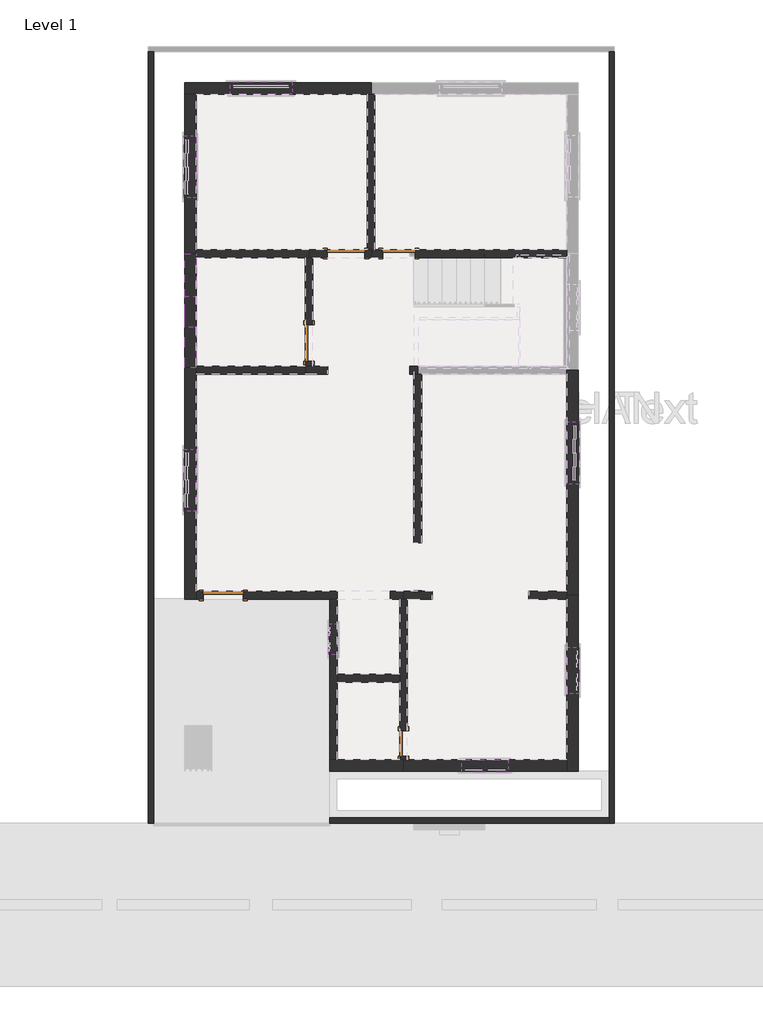
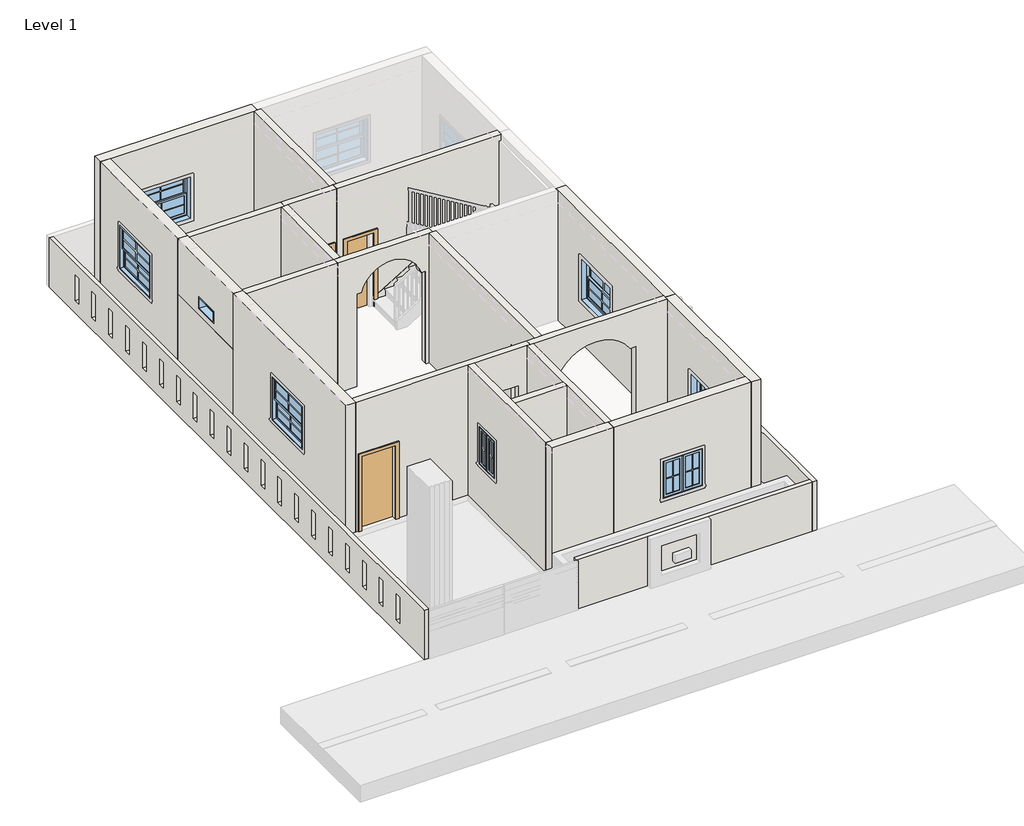
# One storey, part 1 of 3: 25 walls, 8 windows, 5 doors.
"""IFC4 building model written with IfcOpenShell, lengths in millimetres."""

from ifc_helpers import new_model, si_unit, frame, origin, origin_with_axes, place, context, project, spatial, polyline, circle_curve, outline, extrude, faceted_brep, transform, mapped, element, save
from ifc_brep_helpers import plane_surface, revolved_surface, advanced_brep
from components import door_85c31a06, door_fe267433, door_77f51d0b, door_a6948854, door_ee35e093, fixed_2_8c8825d0, window_casement_double_2_fb285ced, window_casement_double_3_90de19e9, window_double_hung_4_eadb0177, window_double_hung_4_aab3aae7

model = new_model("IFC4")

# Units and contexts
model_context = context("Model", 3, world=origin())
ifc_project = project(units=[si_unit("LENGTHUNIT", "METRE", prefix="MILLI")], contexts=[model_context])

# Site, building, storey
site = spatial("IfcSite", under=ifc_project)
building = spatial("IfcBuilding", under=site)
storey = spatial("IfcBuildingStorey", under=building, Name="Level 1", Elevation=0.0)

# Doors
placement = place(None, origin())
door_shape = door_85c31a06(model_context)
element("IfcDoor", 1, ObjectType="Single-Flush : 1'8\"", at=placement, inside=storey, context=model_context, shape_type="MappedRepresentation", body=[
    mapped(door_shape, transform((-1607.764062, -6283.5142637, 152.4), x_axis=(0.0, -1.0, 0.0), y_axis=(1.0, 0.0, 0.0), z_axis=(0.0, 0.0, 1.0))),
])
door_2_shape = door_fe267433(model_context)
element("IfcDoor", 2, ObjectType="Single-Flush : 2'1\"", at=placement, inside=storey, context=model_context, shape_type="MappedRepresentation", body=[
    mapped(door_2_shape, transform((-1696.664062, 3330.3857363, 152.4), x_axis=(-1.0, 0.0, 0.0), y_axis=(0.0, -1.0, 0.0), z_axis=(0.0, 0.0, 1.0))),
])
door_3_shape = door_77f51d0b(model_context)
element("IfcDoor", 3, ObjectType="Single-Flush : 2'4\"", at=placement, inside=storey, context=model_context, shape_type="MappedRepresentation", body=[
    mapped(door_3_shape, transform((-3461.964062, 1577.7857363, 152.4), x_axis=(0.0, -1.0, 0.0), y_axis=(1.0, 0.0, 0.0), z_axis=(0.0, 0.0, 1.0))),
])
door_4_shape = door_a6948854(model_context)
element("IfcDoor", 4, ObjectType="Single-Flush : 2'5\"", at=placement, inside=storey, context=model_context, shape_type="MappedRepresentation", body=[
    mapped(door_4_shape, transform((-2738.064062, 3330.3857363, 152.4), x_axis=(1.0, 0.0, 0.0), y_axis=(0.0, 1.0, 0.0), z_axis=(0.0, 0.0, 1.0))),
])
door_5_shape = door_ee35e093(model_context)
element("IfcDoor", 5, ObjectType="Single-Flush : 2'7\"", at=placement, inside=storey, context=model_context, shape_type="MappedRepresentation", body=[
    mapped(door_5_shape, transform((-5144.714062, -3375.2142637, 152.4), x_axis=(-1.0, 0.0, 0.0), y_axis=(0.0, -1.0, 0.0), z_axis=(0.0, 0.0, 1.0))),
])

# Walls
element("IfcWall", 6, ObjectType="Generic - 4\"", at=placement, inside=storey, context=model_context, shape_type="Brep", body=[
    faceted_brep([(2430.835938, 7292.7857363, 0.0), (2430.835938, -7744.0142637, 0.0), (2430.835938, -7845.6142637, 0.0), (2430.835938, -7845.6142637, 1219.2), (2430.835938, -7744.0142637, 1219.2), (2430.835938, 7292.7857363, 1219.2), (2532.435938, 7292.7857363, 0.0), (2532.435938, 7292.7857363, 1219.2), (2532.435938, -7845.6142637, 1219.2), (2532.435938, -7845.6142637, 0.0)], [[[0, 1, 2, 3, 4, 5]], [[6, 7, 8, 9]], [[2, 1, 0, 6, 9]], [[5, 4, 3, 8, 7]], [[0, 5, 7, 6]], [[3, 2, 9, 8]]]),
])
element("IfcWall", 7, ObjectType="Generic - 4\"", at=placement, inside=storey, context=model_context, shape_type="SweptSolid", body=[
    extrude(outline(polyline([(-3055.564062, -7744.0142637), (2430.835938, -7744.0142637), (2430.835938, -7845.6142637), (-3055.564062, -7845.6142637), (-3055.564062, -7744.0142637)])), origin_with_axes(), (0.0, 0.0, 1.0), 1219.2),
])
element("IfcWall", 8, ObjectType="Generic - 4\"", at=placement, inside=storey, context=model_context, shape_type="SweptSolid", body=[
    extrude(outline(polyline([(7292.7857363, 0.0), (-7845.6142637, 0.0), (-7845.6142637, 1219.2), (7292.7857363, 1219.2), (7292.7857363, 0.0)]), holes=[polyline([(6243.785737, 939.8), (6102.415296, 939.8), (6102.415296, 304.8), (6243.785737, 304.8), (6243.785737, 939.8)]), polyline([(-6722.914263, 939.8), (-6864.284704, 939.8), (-6864.284704, 304.8), (-6722.914263, 304.8), (-6722.914263, 939.8)]), polyline([(-6040.4563683, 939.8), (-6181.8268093, 939.8), (-6181.8268093, 304.8), (-6040.4563683, 304.8), (-6040.4563683, 939.8)]), polyline([(-5357.9984735, 939.8), (-5499.3689146, 939.8), (-5499.3689146, 304.8), (-5357.9984735, 304.8), (-5357.9984735, 939.8)]), polyline([(-4675.5405788, 939.8), (-4816.9110198, 939.8), (-4816.9110198, 304.8), (-4675.5405788, 304.8), (-4675.5405788, 939.8)]), polyline([(-3993.0826841, 939.8), (-4134.4531251, 939.8), (-4134.4531251, 304.8), (-3993.0826841, 304.8), (-3993.0826841, 939.8)]), polyline([(-3310.6247893, 939.8), (-3451.9952303, 939.8), (-3451.9952303, 304.8), (-3310.6247893, 304.8), (-3310.6247893, 939.8)]), polyline([(-2628.1668946, 939.8), (-2769.5373356, 939.8), (-2769.5373356, 304.8), (-2628.1668946, 304.8), (-2628.1668946, 939.8)]), polyline([(-1945.7089999, 939.8), (-2087.0794409, 939.8), (-2087.0794409, 304.8), (-1945.7089999, 304.8), (-1945.7089999, 939.8)]), polyline([(-1263.2511051, 939.8), (-1404.6215461, 939.8), (-1404.6215461, 304.8), (-1263.2511051, 304.8), (-1263.2511051, 939.8)]), polyline([(-580.7932104, 939.8), (-722.1636514, 939.8), (-722.1636514, 304.8), (-580.7932104, 304.8), (-580.7932104, 939.8)]), polyline([(101.6646844, 939.8), (-39.7057567, 939.8), (-39.7057567, 304.8), (101.6646844, 304.8), (101.6646844, 939.8)]), polyline([(784.1225791, 939.8), (642.7521381, 939.8), (642.7521381, 304.8), (784.1225791, 304.8), (784.1225791, 939.8)]), polyline([(1466.5804738, 939.8), (1325.2100328, 939.8), (1325.2100328, 304.8), (1466.5804738, 304.8), (1466.5804738, 939.8)]), polyline([(2149.0383686, 939.8), (2007.6679276, 939.8), (2007.6679276, 304.8), (2149.0383686, 304.8), (2149.0383686, 939.8)]), polyline([(2831.4962633, 939.8), (2690.1258223, 939.8), (2690.1258223, 304.8), (2831.4962633, 304.8), (2831.4962633, 939.8)]), polyline([(3513.954158, 939.8), (3372.583717, 939.8), (3372.583717, 304.8), (3513.954158, 304.8), (3513.954158, 939.8)]), polyline([(4196.4120528, 939.8), (4055.0416118, 939.8), (4055.0416118, 304.8), (4196.4120528, 304.8), (4196.4120528, 939.8)]), polyline([(4878.8699475, 939.8), (4737.4995065, 939.8), (4737.4995065, 304.8), (4878.8699475, 304.8), (4878.8699475, 939.8)]), polyline([(5561.3278422, 939.8), (5419.9574012, 939.8), (5419.9574012, 304.8), (5561.3278422, 304.8), (5561.3278422, 939.8)])]), frame((-6611.564062, 0.0, 0.0), z_axis=(1.0, 0.0, 0.0), x_axis=(0.0, 1.0, 0.0)), (0.0, 0.0, 1.0), 101.6),
])
element("IfcWall", 9, ObjectType="Generic - 6\"", at=placement, inside=storey, context=model_context, shape_type="Brep", body=[
    faceted_brep([(-2318.964062, 6454.5857363, 152.4), (-2318.964062, 3406.5857363, 152.4), (-2318.964062, 3406.5857363, 3352.8), (-2318.964062, 6454.5857363, 3352.8), (-2166.564062, 6454.5857363, 152.4), (-2166.564062, 6454.5857363, 3352.8), (-2166.564062, 3406.5857363, 3352.8), (-2166.564062, 3406.5857363, 152.4), (-2242.764062, 6454.5857363, 152.4), (-2242.764062, 3406.5857363, 152.4), (-2242.764062, 3406.5857363, 3352.8), (-2242.764062, 6454.5857363, 3352.8)], [[[0, 1, 2, 3]], [[4, 5, 6, 7]], [[1, 0, 8, 4, 7, 9]], [[3, 2, 10, 6, 5, 11]], [[0, 3, 11, 5, 4, 8]], [[2, 1, 9, 7, 6, 10]]]),
])
element("IfcWall", 10, ObjectType="Generic - 6\"", at=placement, inside=storey, context=model_context, shape_type="Brep", body=[
    faceted_brep([(-5671.764062, 3254.1857363, 3352.8), (-5671.764062, 3254.1857363, 152.4), (-3538.164062, 3254.1857363, 152.4), (-3461.964062, 3254.1857363, 152.4), (-3461.964062, 3254.1857363, 3352.8), (-3538.164062, 3254.1857363, 3352.8), (-5671.764062, 3406.5857363, 152.4), (-5671.764062, 3406.5857363, 3352.8), (-3461.964062, 3406.5857363, 3352.8), (-3461.964062, 3406.5857363, 152.4), (-5671.764062, 3330.3857363, 152.4), (-5671.764062, 3330.3857363, 3352.8)], [[[0, 1, 2, 3, 4, 5]], [[6, 7, 8, 9]], [[3, 2, 1, 10, 6, 9]], [[4, 3, 9, 8]], [[0, 5, 4, 8, 7, 11]], [[0, 11, 7, 6, 10, 1]]]),
])
element("IfcWall", 11, ObjectType="Generic - 6\"", at=placement, inside=storey, context=model_context, shape_type="Brep", body=[
    faceted_brep([(-5671.764062, 968.1857363, 152.4), (-3538.164062, 968.1857363, 152.4), (-3538.164062, 968.1857363, 3352.8), (-5671.764062, 968.1857363, 3352.8), (-5671.764062, 1120.5857363, 152.4), (-5671.764062, 1120.5857363, 3352.8), (-3538.164062, 1120.5857363, 3352.8), (-3538.164062, 1120.5857363, 152.4), (-5671.764062, 1095.1857363, 152.4), (-5671.764062, 1095.1857363, 3352.8)], [[[0, 1, 2, 3]], [[4, 5, 6, 7]], [[1, 0, 8, 4, 7]], [[2, 1, 7, 6]], [[3, 2, 6, 5, 9]], [[0, 3, 9, 5, 4, 8]]]),
])
element("IfcWall", 12, ObjectType="Generic - 6\"", at=placement, inside=storey, context=model_context, shape_type="Brep", body=[
    faceted_brep([(-1404.564062, 968.1857363, 152.4), (-1404.564062, -2346.4297845, 152.4), (-1404.564062, -2346.4297845, 2616.2), (-1404.564062, -3288.7710229, 2616.2), (-1404.564062, -3288.7710229, 152.4), (-1404.564062, -3299.0142637, 152.4), (-1404.564062, -3299.0142637, 3352.8), (-1404.564062, 968.1857363, 3352.8), (-1252.164062, -2346.4297845, 152.4), (-1252.164062, 968.1857363, 152.4), (-1252.164062, 968.1857363, 3352.8), (-1252.164062, -3299.0142637, 3352.8), (-1252.164062, -3299.0142637, 152.4), (-1252.164062, -3288.7710229, 152.4), (-1252.164062, -3288.7710229, 2616.2), (-1252.164062, -2346.4297845, 2616.2), (-1328.364062, 968.1857363, 152.4), (-1328.364062, 968.1857363, 3352.8)], [[[0, 1, 2, 3, 4, 5, 6, 7]], [[8, 9, 10, 11, 12, 13, 14, 15]], [[6, 5, 12, 11]], [[1, 0, 16, 9, 8]], [[7, 6, 11, 10, 17]], [[2, 1, 8, 15]], [[3, 2, 15, 14]], [[4, 3, 14, 13]], [[5, 4, 13, 12]], [[0, 7, 17, 10, 9, 16]]]),
])
element("IfcWall", 13, ObjectType="Generic - 6\"", at=placement, inside=storey, context=model_context, shape_type="Brep", body=[
    faceted_brep([(-2903.164062, -3451.4142637, 2438.4), (-1865.8319448, -3451.4142637, 2438.4), (-1865.8319448, -3451.4142637, 152.4), (-1683.964062, -3451.4142637, 152.4), (-1607.764062, -3451.4142637, 152.4), (-1607.764062, -3451.4142637, 3352.8), (-1683.964062, -3451.4142637, 3352.8), (-2903.164062, -3451.4142637, 3352.8), (-3055.564062, -3451.4142637, 3352.8), (-5671.764062, -3451.4142637, 3352.8), (-5671.764062, -3451.4142637, 152.4), (-5538.414062, -3451.4142637, 152.4), (-5538.414062, -3451.4142637, 1981.2), (-4751.014062, -3451.4142637, 1981.2), (-4751.014062, -3451.4142637, 152.4), (-3055.564062, -3451.4142637, 152.4), (-2903.164062, -3451.4142637, 152.4), (-1865.8319448, -3299.0142637, 2438.4), (-2903.164062, -3299.0142637, 2438.4), (-2903.164062, -3299.0142637, 152.4), (-4751.014062, -3299.0142637, 152.4), (-4751.014062, -3299.0142637, 1981.2), (-5538.414062, -3299.0142637, 1981.2), (-5538.414062, -3299.0142637, 152.4), (-5671.764062, -3299.0142637, 152.4), (-5671.764062, -3299.0142637, 3352.8), (-1607.764062, -3299.0142637, 3352.8), (-1607.764062, -3299.0142637, 152.4), (-1865.8319448, -3299.0142637, 152.4)], [[[0, 1, 2, 3, 4, 5, 6, 7, 8, 9, 10, 11, 12, 13, 14, 15, 16]], [[17, 18, 19, 20, 21, 22, 23, 24, 25, 26, 27, 28]], [[17, 1, 0, 18]], [[1, 17, 28, 2]], [[22, 12, 11, 23]], [[12, 22, 21, 13]], [[13, 21, 20, 14]], [[10, 24, 23, 11]], [[27, 4, 3, 2, 28]], [[19, 16, 15, 14, 20]], [[5, 4, 27, 26]], [[9, 8, 7, 6, 5, 26, 25]], [[10, 9, 25, 24]], [[18, 0, 16, 19]]]),
])
element("IfcWall", 14, ObjectType="Generic - 6\"", at=placement, inside=storey, context=model_context, shape_type="Brep", body=[
    faceted_brep([(-3055.564062, -3451.4142637, 152.4), (-3055.564062, -6601.0142637, 152.4), (-3055.564062, -6601.0142637, 3352.8), (-3055.564062, -3451.4142637, 3352.8), (-3055.564062, -3934.0142637, 2133.6), (-3055.564062, -4543.6142637, 2133.6), (-3055.564062, -4543.6142637, 1219.2), (-3055.564062, -3934.0142637, 1219.2), (-2903.164062, -3451.4142637, 152.4), (-2903.164062, -3451.4142637, 2438.4), (-2903.164062, -3451.4142637, 3352.8), (-2903.164062, -4924.6142637, 3352.8), (-2903.164062, -5077.0142637, 3352.8), (-2903.164062, -6601.0142637, 3352.8), (-2903.164062, -6601.0142637, 152.4), (-2903.164062, -5077.0142637, 152.4), (-2903.164062, -4924.6142637, 152.4), (-2903.164062, -3934.0142637, 2133.6), (-2903.164062, -3934.0142637, 1219.2), (-2903.164062, -4543.6142637, 1219.2), (-2903.164062, -4543.6142637, 2133.6)], [[[0, 1, 2, 3], [4, 5, 6, 7]], [[8, 9, 10, 11, 12, 13, 14, 15, 16], [17, 18, 19, 20]], [[1, 0, 8, 16, 15, 14]], [[3, 2, 13, 12, 11, 10]], [[2, 1, 14, 13]], [[18, 17, 4, 7]], [[19, 18, 7, 6]], [[20, 19, 6, 5]], [[17, 20, 5, 4]], [[0, 3, 10, 9, 8]]]),
])
element("IfcWall", 15, ObjectType="Generic - 6\"", at=placement, inside=storey, context=model_context, shape_type="Brep", body=[
    faceted_brep([(-1683.964062, -6601.0142637, 3352.8), (-1683.964062, -5077.0142637, 3352.8), (-1683.964062, -4924.6142637, 3352.8), (-1683.964062, -3451.4142637, 3352.8), (-1683.964062, -3451.4142637, 152.4), (-1683.964062, -4924.6142637, 152.4), (-1683.964062, -5077.0142637, 152.4), (-1683.964062, -6029.5142637, 152.4), (-1683.964062, -6029.5142637, 1981.2), (-1683.964062, -6537.5142637, 1981.2), (-1683.964062, -6537.5142637, 152.4), (-1683.964062, -6601.0142637, 152.4), (-1531.564062, -3451.4142637, 3352.8), (-1531.564062, -6601.0142637, 3352.8), (-1531.564062, -6601.0142637, 152.4), (-1531.564062, -6537.5142637, 152.4), (-1531.564062, -6537.5142637, 1981.2), (-1531.564062, -6029.5142637, 1981.2), (-1531.564062, -6029.5142637, 152.4), (-1531.564062, -3451.4142637, 152.4), (-1607.764062, -6601.0142637, 152.4), (-1607.764062, -3451.4142637, 152.4), (-1607.764062, -6601.0142637, 3352.8), (-1607.764062, -3451.4142637, 3352.8)], [[[0, 1, 2, 3, 4, 5, 6, 7, 8, 9, 10, 11]], [[12, 13, 14, 15, 16, 17, 18, 19]], [[14, 20, 11, 10, 15]], [[4, 21, 19, 18, 7, 6, 5]], [[3, 2, 1, 0, 22, 13, 12, 23]], [[9, 16, 15, 10]], [[16, 9, 8, 17]], [[17, 8, 7, 18]], [[0, 11, 20, 14, 13, 22]], [[4, 3, 23, 12, 19, 21]]]),
])
element("IfcWall", 16, ObjectType="Generic - 6\"", at=placement, inside=storey, context=model_context, shape_type="SweptSolid", body=[
    extrude(outline(polyline([(-1683.964062, -5077.0142637), (-2903.164062, -5077.0142637), (-2903.164062, -4924.6142637), (-1683.964062, -4924.6142637), (-1683.964062, -5077.0142637)])), frame((0.0, 0.0, 152.4), z_axis=(0.0, 0.0, 1.0), x_axis=(1.0, 0.0, 0.0)), (0.0, 0.0, 1.0), 3200.4),
])
element("IfcWall", 17, ObjectType="Generic - 6\"", at=placement, inside=storey, context=model_context, shape_type="Brep", body=[
    faceted_brep([(-3538.164062, 1120.5857363, 3352.8), (-3538.164062, 3254.1857363, 3352.8), (-3538.164062, 3254.1857363, 152.4), (-3538.164062, 1933.3857363, 152.4), (-3538.164062, 1933.3857363, 1981.2), (-3538.164062, 1222.1857363, 1981.2), (-3538.164062, 1222.1857363, 152.4), (-3538.164062, 1120.5857363, 152.4), (-3385.764062, 3254.1857363, 3352.8), (-3385.764062, 1120.5857363, 3352.8), (-3385.764062, 1120.5857363, 152.4), (-3385.764062, 1222.1857363, 152.4), (-3385.764062, 1222.1857363, 1981.2), (-3385.764062, 1933.3857363, 1981.2), (-3385.764062, 1933.3857363, 152.4), (-3385.764062, 3254.1857363, 152.4), (-3461.964062, 3254.1857363, 152.4), (-3461.964062, 3254.1857363, 3352.8)], [[[0, 1, 2, 3, 4, 5, 6, 7]], [[8, 9, 10, 11, 12, 13, 14, 15]], [[10, 7, 6, 11]], [[2, 16, 15, 14, 3]], [[1, 0, 9, 8, 17]], [[0, 7, 10, 9]], [[12, 5, 4, 13]], [[13, 4, 3, 14]], [[5, 12, 11, 6]], [[2, 1, 17, 8, 15, 16]]]),
])
element("IfcWall", 18, ObjectType="Generic - 6\"", at=placement, inside=storey, context=model_context, shape_type="Brep", body=[
    faceted_brep([(-2242.764062, 3254.1857363, 152.4), (-2014.164062, 3254.1857363, 152.4), (-2014.164062, 3254.1857363, 1981.2), (-1379.164062, 3254.1857363, 1981.2), (-1379.164062, 3254.1857363, 152.4), (1541.835938, 3254.1857363, 152.4), (1592.635938, 3254.1857363, 152.4), (1592.635938, 3254.1857363, 3352.8), (-2242.764062, 3254.1857363, 3352.8), (-2014.164062, 3406.5857363, 1981.2), (-2014.164062, 3406.5857363, 152.4), (-2166.564062, 3406.5857363, 152.4), (-2242.764062, 3406.5857363, 152.4), (-2242.764062, 3406.5857363, 3352.8), (-2166.564062, 3406.5857363, 3352.8), (1592.635938, 3406.5857363, 3352.8), (1592.635938, 3406.5857363, 152.4), (-1379.164062, 3406.5857363, 152.4), (-1379.164062, 3406.5857363, 1981.2), (1592.635938, 3330.3857363, 152.4), (1592.635938, 3330.3857363, 3352.8)], [[[0, 1, 2, 3, 4, 5, 6, 7, 8]], [[9, 10, 11, 12, 13, 14, 15, 16, 17, 18]], [[17, 16, 19, 6, 5, 4]], [[12, 11, 10, 1, 0]], [[8, 7, 20, 15, 14, 13]], [[0, 8, 13, 12]], [[4, 3, 18, 17]], [[3, 2, 9, 18]], [[2, 1, 10, 9]], [[6, 19, 16, 15, 20, 7]]]),
])
element("IfcWall", 19, ObjectType="Generic - 6\"", at=placement, inside=storey, context=model_context, shape_type="AdvancedBrep", body=[
    advanced_brep(
    [(1592.635938, -3451.4142637, 3352.8), (-1531.564062, -3451.4142637, 3352.8), (-1607.764062, -3451.4142637, 3352.8), (-1607.764062, -3451.4142637, 152.4), (-1531.564062, -3451.4142637, 152.4), (-1042.9877715, -3451.4142637, 152.4), (-1042.9877715, -3451.4142637, 2438.4), (-909.3649468, -3451.4142637, 2438.4), (732.5205767, -3451.4142637, 2438.4), (852.655246, -3451.4142637, 2438.4), (852.655246, -3451.4142637, 152.4), (1592.635938, -3451.4142637, 152.4), (-1607.764062, -3299.0142637, 3352.8), (-1404.564062, -3299.0142637, 3352.8), (-1252.164062, -3299.0142637, 3352.8), (1592.635938, -3299.0142637, 3352.8), (1592.635938, -3299.0142637, 152.4), (852.655246, -3299.0142637, 152.4), (852.655246, -3299.0142637, 2438.4), (732.5205767, -3299.0142637, 2438.4), (-909.3649468, -3299.0142637, 2438.4), (-1042.9877715, -3299.0142637, 2438.4), (-1042.9877715, -3299.0142637, 152.4), (-1252.164062, -3299.0142637, 152.4), (-1404.564062, -3299.0142637, 152.4), (-1607.764062, -3299.0142637, 152.4), (1592.635938, -3375.2142637, 3352.8), (1592.635938, -3375.2142637, 152.4)],
    [
        (0, 1),
        (1, 2),
        (2, 3),
        (3, 4),
        (4, 5),
        (5, 6),
        (6, 7),
        (7, 8, circle_curve(frame((-88.4221851, -3451.4142637, 1902.6141821), z_axis=(0.0, 1.0, 0.0), x_axis=(-1.0, 0.0, 0.0)), 980.3129402)),
        (8, 9),
        (9, 10),
        (10, 11),
        (11, 0),
        (12, 13),
        (13, 14),
        (14, 15),
        (15, 16),
        (16, 17),
        (17, 18),
        (18, 19),
        (19, 20, circle_curve(frame((-88.4221851, -3299.0142637, 1902.6141821), z_axis=(0.0, -1.0, 0.0), x_axis=(-1.0, 0.0, 0.0)), 980.3129402)),
        (20, 21),
        (21, 22),
        (22, 23),
        (23, 24),
        (24, 25),
        (25, 12),
        (0, 26),
        (26, 15),
        (12, 2),
        (9, 18),
        (17, 10),
        (5, 22),
        (21, 6),
        (7, 20),
        (19, 8),
        (3, 25),
        (16, 27),
        (27, 11),
    ],
    [
        plane_surface(frame((1706.935938, -3451.4142637, 3352.8), z_axis=(0.0, -1.0, 0.0), x_axis=(-1.0, 0.0, 0.0))),
        plane_surface(frame((1706.935938, -3299.0142637, 3352.8), z_axis=(0.0, 1.0, 0.0), x_axis=(1.0, 0.0, 0.0))),
        plane_surface(frame((1706.935938, -3451.4142637, 3352.8), z_axis=(0.0, 0.0, 1.0), x_axis=(0.0, 1.0, 0.0))),
        plane_surface(frame((852.655246, -3451.4142637, 2177.180621), z_axis=(-1.0, 0.0, 0.0), x_axis=(0.0, 1.0, 0.0))),
        plane_surface(frame((-1042.9877715, -3451.4142637, 487.9784957), z_axis=(1.0, 0.0, 0.0), x_axis=(0.0, 1.0, 0.0))),
        revolved_surface(polyline([(-1068.7351253, -3299.0142637, 1902.6141821), (-1068.7351253, -3451.4142637, 1902.6141821)]), (-88.4221851, -3299.0142637, 1902.6141821), (0.0, 1.0, 0.0)),
        plane_surface(frame((-1607.764062, -3451.4142637, 152.4), z_axis=(0.0, 0.0, -1.0), x_axis=(0.0, 1.0, 0.0))),
        plane_surface(frame((456.9071606, -3451.4142637, 152.4), z_axis=(0.0, 0.0, -1.0), x_axis=(0.0, 1.0, 0.0))),
        plane_surface(frame((-1607.764062, -3451.4142637, 3352.8), z_axis=(-1.0, 0.0, 0.0), x_axis=(0.0, 1.0, 0.0))),
        plane_surface(frame((1592.635938, 6454.5857363, 152.4), z_axis=(1.0, 0.0, 0.0), x_axis=(0.0, -1.0, 0.0))),
        plane_surface(frame((-1042.9877715, -3299.0142637, 2438.4), z_axis=(0.0, 0.0, -1.0), x_axis=(-1.0, 0.0, 0.0))),
    ],
    [
        (0, [[1, 2, 3, 4, 5, 6, 7, 8, 9, 10, 11, 12]]),
        (1, [[13, 14, 15, 16, 17, 18, 19, 20, 21, 22, 23, 24, 25, 26]]),
        (2, [[-2, -1, 27, 28, -15, -14, -13, 29]]),
        (3, [[30, -18, 31, -10]]),
        (4, [[32, -22, 33, -6]]),
        (5, [[-8, 34, -20, 35]]),
        (6, [[36, -25, -24, -23, -32, -5, -4]]),
        (7, [[37, 38, -11, -31, -17]]),
        (8, [[-3, -29, -26, -36]]),
        (9, [[-12, -38, -37, -16, -28, -27]]),
        (10, [[-33, -21, -34, -7]]),
        (10, [[-30, -9, -35, -19]]),
    ],
),
])
element("IfcWall", 20, ObjectType="Generic - 6\"", at=placement, inside=storey, context=model_context, shape_type="Brep", body=[
    faceted_brep([(-2369.764062, 3254.1857363, 1981.2), (-2369.764062, 3254.1857363, 152.4), (-2242.764062, 3254.1857363, 152.4), (-2242.764062, 3254.1857363, 3352.8), (-3385.764062, 3254.1857363, 3352.8), (-3461.964062, 3254.1857363, 3352.8), (-3461.964062, 3254.1857363, 152.4), (-3385.764062, 3254.1857363, 152.4), (-3106.364062, 3254.1857363, 152.4), (-3106.364062, 3254.1857363, 1981.2), (-2242.764062, 3406.5857363, 152.4), (-2318.964062, 3406.5857363, 152.4), (-2369.764062, 3406.5857363, 152.4), (-2369.764062, 3406.5857363, 1981.2), (-3106.364062, 3406.5857363, 1981.2), (-3106.364062, 3406.5857363, 152.4), (-3461.964062, 3406.5857363, 152.4), (-3461.964062, 3406.5857363, 3352.8), (-2318.964062, 3406.5857363, 3352.8), (-2242.764062, 3406.5857363, 3352.8)], [[[0, 1, 2, 3, 4, 5, 6, 7, 8, 9]], [[10, 11, 12, 13, 14, 15, 16, 17, 18, 19]], [[2, 1, 12, 11, 10]], [[8, 7, 6, 16, 15]], [[3, 2, 10, 19]], [[5, 4, 3, 19, 18, 17]], [[6, 5, 17, 16]], [[15, 14, 9, 8]], [[14, 13, 0, 9]], [[13, 12, 1, 0]]]),
])
element("IfcWall", 21, ObjectType="Generic - 6\"", at=placement, inside=storey, context=model_context, shape_type="AdvancedBrep", body=[
    advanced_brep(
    [(-1328.364062, 968.1857363, 3352.8), (-1404.564062, 968.1857363, 3352.8), (-3538.164062, 968.1857363, 3352.8), (-3538.164062, 968.1857363, 152.4), (-3088.5741654, 968.1857363, 152.4), (-3088.5741654, 968.1857363, 2438.4), (-2990.069581, 968.1857363, 2438.4), (-1595.0493956, 968.1857363, 2438.4), (-1480.764062, 968.1857363, 2438.4), (-1480.764062, 968.1857363, 152.4), (-1404.564062, 968.1857363, 152.4), (-1328.364062, 968.1857363, 152.4), (-3538.164062, 1120.5857363, 3352.8), (-3385.764062, 1120.5857363, 3352.8), (-1328.364062, 1120.5857363, 3352.8), (-1328.364062, 1120.5857363, 152.4), (-1480.764062, 1120.5857363, 152.4), (-1480.764062, 1120.5857363, 2438.4), (-1595.0493956, 1120.5857363, 2438.4), (-2990.069581, 1120.5857363, 2438.4), (-3088.5741654, 1120.5857363, 2438.4), (-3088.5741654, 1120.5857363, 152.4), (-3385.764062, 1120.5857363, 152.4), (-3538.164062, 1120.5857363, 152.4)],
    [
        (0, 1),
        (1, 2),
        (2, 3),
        (3, 4),
        (4, 5),
        (5, 6),
        (6, 7, circle_curve(frame((-2292.5594883, 968.1857363, 2260.6), z_axis=(0.0, 1.0, 0.0), x_axis=(-1.0, 0.0, 0.0)), 719.8146771)),
        (7, 8),
        (8, 9),
        (9, 10),
        (10, 11),
        (11, 0),
        (12, 13),
        (13, 14),
        (14, 15),
        (15, 16),
        (16, 17),
        (17, 18),
        (18, 19, circle_curve(frame((-2292.5594883, 1120.5857363, 2260.6), z_axis=(0.0, -1.0, 0.0), x_axis=(-1.0, 0.0, 0.0)), 719.8146771)),
        (19, 20),
        (20, 21),
        (21, 22),
        (22, 23),
        (23, 12),
        (6, 19),
        (18, 7),
        (15, 11),
        (9, 16),
        (0, 14),
        (12, 2),
        (3, 23),
        (21, 4),
        (5, 20),
        (17, 8),
    ],
    [
        plane_surface(frame((-3012.3741654, 968.1857363, 2260.6), z_axis=(0.0, -1.0, 0.0), x_axis=(0.0, 0.0, 1.0))),
        plane_surface(frame((-3012.3741654, 1120.5857363, 2260.6), z_axis=(0.0, 1.0, 0.0), x_axis=(0.0, 0.0, -1.0))),
        revolved_surface(polyline([(-3012.3741654, 1120.5857363, 2260.6), (-3012.3741654, 968.1857363, 2260.6)]), (-2292.5594883, 1120.5857363, 2260.6), (0.0, 1.0, 0.0)),
        plane_surface(frame((-1572.7448112, 968.1857363, 152.4), z_axis=(0.0, 0.0, -1.0), x_axis=(0.0, 1.0, 0.0))),
        plane_surface(frame((-1328.364062, 968.1857363, 3352.8), z_axis=(0.0, 0.0, 1.0), x_axis=(0.0, 1.0, 0.0))),
        plane_surface(frame((-3538.164062, 968.1857363, 152.4), z_axis=(0.0, 0.0, -1.0), x_axis=(0.0, 1.0, 0.0))),
        plane_surface(frame((-1328.364062, 968.1857363, 152.4), z_axis=(1.0, 0.0, 0.0), x_axis=(0.0, 1.0, 0.0))),
        plane_surface(frame((-3538.164062, 968.1857363, 3352.8), z_axis=(-1.0, 0.0, 0.0), x_axis=(0.0, 1.0, 0.0))),
        plane_surface(frame((-3088.5741654, 1120.5857363, 2438.4), z_axis=(0.0, 0.0, -1.0), x_axis=(-1.0, 0.0, 0.0))),
        plane_surface(frame((-3088.5741654, 1120.5857363, 2438.4), z_axis=(1.0, 0.0, 0.0), x_axis=(0.0, 0.0, -1.0))),
        plane_surface(frame((-1480.764062, 968.1857363, 2438.4), z_axis=(-1.0, 0.0, 0.0), x_axis=(0.0, 0.0, -1.0))),
    ],
    [
        (0, [[1, 2, 3, 4, 5, 6, 7, 8, 9, 10, 11, 12]]),
        (1, [[13, 14, 15, 16, 17, 18, 19, 20, 21, 22, 23, 24]]),
        (2, [[-7, 25, -19, 26]]),
        (3, [[27, -11, -10, 28, -16]]),
        (4, [[-2, -1, 29, -14, -13, 30]]),
        (5, [[31, -23, -22, 32, -4]]),
        (6, [[-12, -27, -15, -29]]),
        (7, [[-3, -30, -24, -31]]),
        (8, [[33, -20, -25, -6]]),
        (8, [[34, -8, -26, -18]]),
        (9, [[-33, -5, -32, -21]]),
        (10, [[-34, -17, -28, -9]]),
    ],
),
])
element("IfcWall", 22, ObjectType="Generic - 9\"", at=placement, inside=storey, context=model_context, shape_type="Brep", body=[
    faceted_brep([(-5900.364062, 6454.5857363, 152.4), (-5671.764062, 6454.5857363, 152.4), (-2318.964062, 6454.5857363, 152.4), (-2242.764062, 6454.5857363, 152.4), (-2242.764062, 6454.5857363, 3352.8), (-2318.964062, 6454.5857363, 3352.8), (-5671.764062, 6454.5857363, 3352.8), (-5900.364062, 6454.5857363, 3352.8), (-3792.164062, 6454.5857363, 2286.0), (-3792.164062, 6454.5857363, 1219.2), (-5011.364062, 6454.5857363, 1219.2), (-5011.364062, 6454.5857363, 2286.0), (-5900.364062, 6683.1857363, 152.4), (-5900.364062, 6683.1857363, 3352.8), (-2242.764062, 6683.1857363, 3352.8), (-2242.764062, 6683.1857363, 152.4), (-3792.164062, 6683.1857363, 2286.0), (-5011.364062, 6683.1857363, 2286.0), (-5011.364062, 6683.1857363, 1219.2), (-3792.164062, 6683.1857363, 1219.2)], [[[0, 1, 2, 3, 4, 5, 6, 7], [8, 9, 10, 11]], [[12, 13, 14, 15], [16, 17, 18, 19]], [[3, 2, 1, 0, 12, 15]], [[4, 3, 15, 14]], [[7, 6, 5, 4, 14, 13]], [[0, 7, 13, 12]], [[9, 8, 16, 19]], [[10, 9, 19, 18]], [[11, 10, 18, 17]], [[8, 11, 17, 16]]]),
])
element("IfcWall", 23, ObjectType="Generic - 9\"", at=placement, inside=storey, context=model_context, shape_type="Brep", body=[
    faceted_brep([(1592.635938, -6601.0142637, 152.4), (-1531.564062, -6601.0142637, 152.4), (-1607.764062, -6601.0142637, 152.4), (-1607.764062, -6601.0142637, 3352.8), (-1531.564062, -6601.0142637, 3352.8), (1592.635938, -6601.0142637, 3352.8), (-464.764062, -6601.0142637, 2133.6), (-464.764062, -6601.0142637, 1219.2), (449.635938, -6601.0142637, 1219.2), (449.635938, -6601.0142637, 2133.6), (1592.635938, -6829.6142637, 152.4), (1592.635938, -6829.6142637, 3352.8), (-1607.764062, -6829.6142637, 3352.8), (-1607.764062, -6829.6142637, 152.4), (-464.764062, -6829.6142637, 2133.6), (449.635938, -6829.6142637, 2133.6), (449.635938, -6829.6142637, 1219.2), (-464.764062, -6829.6142637, 1219.2)], [[[0, 1, 2, 3, 4, 5], [6, 7, 8, 9]], [[10, 11, 12, 13], [14, 15, 16, 17]], [[2, 1, 0, 10, 13]], [[3, 2, 13, 12]], [[5, 4, 3, 12, 11]], [[0, 5, 11, 10]], [[7, 6, 14, 17]], [[8, 7, 17, 16]], [[9, 8, 16, 15]], [[6, 9, 15, 14]]]),
])
element("IfcWall", 24, ObjectType="Generic - 9\"", at=placement, inside=storey, context=model_context, shape_type="Brep", body=[
    faceted_brep([(-5900.364062, 6454.5857363, 152.4), (-5900.364062, 3330.3857363, 152.4), (-5900.364062, 3330.3857363, 1981.2), (-5900.364062, 3330.3857363, 3352.8), (-5900.364062, 6454.5857363, 3352.8), (-5900.364062, 4422.5857363, 2286.0), (-5900.364062, 4422.5857363, 1219.2), (-5900.364062, 5641.7857363, 1219.2), (-5900.364062, 5641.7857363, 2286.0), (-5671.764062, 6454.5857363, 152.4), (-5671.764062, 6454.5857363, 3352.8), (-5671.764062, 3406.5857363, 3352.8), (-5671.764062, 3330.3857363, 3352.8), (-5671.764062, 3330.3857363, 152.4), (-5671.764062, 3406.5857363, 152.4), (-5671.764062, 4422.5857363, 2286.0), (-5671.764062, 5641.7857363, 2286.0), (-5671.764062, 5641.7857363, 1219.2), (-5671.764062, 4422.5857363, 1219.2)], [[[0, 1, 2, 3, 4], [5, 6, 7, 8]], [[9, 10, 11, 12, 13, 14], [15, 16, 17, 18]], [[1, 0, 9, 14, 13]], [[4, 3, 12, 11, 10]], [[0, 4, 10, 9]], [[6, 5, 15, 18]], [[7, 6, 18, 17]], [[8, 7, 17, 16]], [[5, 8, 16, 15]], [[1, 13, 12, 3, 2]]]),
])
element("IfcWall", 25, ObjectType="Generic - 9\"", at=placement, inside=storey, context=model_context, shape_type="Brep", body=[
    faceted_brep([(-5900.364062, 3330.3857363, 152.4), (-5900.364062, 1095.1857363, 152.4), (-5900.364062, 1095.1857363, 1981.2), (-5900.364062, 3330.3857363, 1981.2), (-5671.764062, 3330.3857363, 152.4), (-5671.764062, 3330.3857363, 1981.2), (-5671.764062, 1095.1857363, 1981.2), (-5671.764062, 1095.1857363, 152.4), (-5671.764062, 3254.1857363, 152.4)], [[[0, 1, 2, 3]], [[4, 5, 6, 7, 8]], [[1, 0, 4, 8, 7]], [[2, 1, 7, 6]], [[3, 2, 6, 5]], [[0, 3, 5, 4]]]),
])
element("IfcWall", 26, ObjectType="Generic - 9\"", at=placement, inside=storey, context=model_context, shape_type="Brep", body=[
    faceted_brep([(-1607.764062, -6601.0142637, 152.4), (-1683.964062, -6601.0142637, 152.4), (-2903.164062, -6601.0142637, 152.4), (-3055.564062, -6601.0142637, 152.4), (-3055.564062, -6601.0142637, 3352.8), (-2903.164062, -6601.0142637, 3352.8), (-1683.964062, -6601.0142637, 3352.8), (-1607.764062, -6601.0142637, 3352.8), (-1607.764062, -6829.6142637, 152.4), (-1607.764062, -6829.6142637, 3352.8), (-3055.564062, -6829.6142637, 3352.8), (-3055.564062, -6829.6142637, 152.4)], [[[0, 1, 2, 3, 4, 5, 6, 7]], [[8, 9, 10, 11]], [[3, 2, 1, 0, 8, 11]], [[7, 6, 5, 4, 10, 9]], [[0, 7, 9, 8]], [[4, 3, 11, 10]]]),
])
element("IfcWall", 27, ObjectType="Generic - 9\"", at=placement, inside=storey, context=model_context, shape_type="Brep", body=[
    faceted_brep([(1592.635938, 1044.3857363, 3352.8), (1592.635938, 1044.3857363, 152.4), (1592.635938, 993.5857363, 152.4), (1592.635938, 968.1857363, 152.4), (1592.635938, -3299.0142637, 152.4), (1592.635938, -3375.2142637, 152.4), (1592.635938, -3375.2142637, 3352.8), (1592.635938, -3299.0142637, 3352.8), (1592.635938, 968.1857363, 3352.8), (1592.635938, 28.3857363, 2286.0), (1592.635938, -1190.8142637, 2286.0), (1592.635938, -1190.8142637, 1219.2), (1592.635938, 28.3857363, 1219.2), (1821.235938, 1044.3857363, 152.4), (1821.235938, 1044.3857363, 3352.8), (1821.235938, -3375.2142637, 3352.8), (1821.235938, -3375.2142637, 152.4), (1821.235938, 28.3857363, 2286.0), (1821.235938, 28.3857363, 1219.2), (1821.235938, -1190.8142637, 1219.2), (1821.235938, -1190.8142637, 2286.0)], [[[0, 1, 2, 3, 4, 5, 6, 7, 8], [9, 10, 11, 12]], [[13, 14, 15, 16], [17, 18, 19, 20]], [[5, 4, 3, 2, 1, 13, 16]], [[6, 5, 16, 15]], [[0, 8, 7, 6, 15, 14]], [[17, 20, 10, 9]], [[20, 19, 11, 10]], [[19, 18, 12, 11]], [[18, 17, 9, 12]], [[0, 14, 13, 1]]]),
])
element("IfcWall", 28, ObjectType="Generic - 9\"", at=placement, inside=storey, context=model_context, shape_type="Brep", body=[
    faceted_brep([(1592.635938, -3375.2142637, 152.4), (1592.635938, -3451.4142637, 152.4), (1592.635938, -6601.0142637, 152.4), (1592.635938, -6829.6142637, 152.4), (1592.635938, -6829.6142637, 3352.8), (1592.635938, -6601.0142637, 3352.8), (1592.635938, -3451.4142637, 3352.8), (1592.635938, -3375.2142637, 3352.8), (1592.635938, -5305.6142637, 2133.6), (1592.635938, -5305.6142637, 1219.2), (1592.635938, -4391.2142637, 1219.2), (1592.635938, -4391.2142637, 2133.6), (1821.235938, -3375.2142637, 152.4), (1821.235938, -3375.2142637, 3352.8), (1821.235938, -6829.6142637, 3352.8), (1821.235938, -6829.6142637, 152.4), (1821.235938, -5305.6142637, 2133.6), (1821.235938, -4391.2142637, 2133.6), (1821.235938, -4391.2142637, 1219.2), (1821.235938, -5305.6142637, 1219.2)], [[[0, 1, 2, 3, 4, 5, 6, 7], [8, 9, 10, 11]], [[12, 13, 14, 15], [16, 17, 18, 19]], [[3, 2, 1, 0, 12, 15]], [[7, 6, 5, 4, 14, 13]], [[0, 7, 13, 12]], [[4, 3, 15, 14]], [[8, 11, 17, 16]], [[11, 10, 18, 17]], [[10, 9, 19, 18]], [[9, 8, 16, 19]]]),
])
element("IfcWall", 29, ObjectType="Generic - 9\"", at=placement, inside=storey, context=model_context, shape_type="Brep", body=[
    faceted_brep([(-5900.364062, 1095.1857363, 3352.8), (-5900.364062, 1095.1857363, 1981.2), (-5900.364062, 1095.1857363, 152.4), (-5900.364062, -3451.4142637, 152.4), (-5900.364062, -3451.4142637, 3352.8), (-5900.364062, -1724.2142637, 2286.0), (-5900.364062, -1724.2142637, 1219.2), (-5900.364062, -505.0142637, 1219.2), (-5900.364062, -505.0142637, 2286.0), (-5671.764062, 1095.1857363, 152.4), (-5671.764062, 1095.1857363, 1981.2), (-5671.764062, 1095.1857363, 3352.8), (-5671.764062, 968.1857363, 3352.8), (-5671.764062, -3299.0142637, 3352.8), (-5671.764062, -3451.4142637, 3352.8), (-5671.764062, -3451.4142637, 152.4), (-5671.764062, -3299.0142637, 152.4), (-5671.764062, 968.1857363, 152.4), (-5671.764062, -1724.2142637, 2286.0), (-5671.764062, -505.0142637, 2286.0), (-5671.764062, -505.0142637, 1219.2), (-5671.764062, -1724.2142637, 1219.2)], [[[0, 1, 2, 3, 4], [5, 6, 7, 8]], [[9, 10, 11, 12, 13, 14, 15, 16, 17], [18, 19, 20, 21]], [[3, 2, 9, 17, 16, 15]], [[0, 4, 14, 13, 12, 11]], [[4, 3, 15, 14]], [[5, 8, 19, 18]], [[8, 7, 20, 19]], [[7, 6, 21, 20]], [[6, 5, 18, 21]], [[0, 11, 10, 9, 2, 1]]]),
])
element("IfcWall", 30, ObjectType="Generic - 9\"", at=placement, inside=storey, context=model_context, shape_type="Brep", body=[
    faceted_brep([(-5900.364062, 3330.3857363, 1981.2), (-5900.364062, 1095.1857363, 1981.2), (-5900.364062, 1095.1857363, 3352.8), (-5900.364062, 3330.3857363, 3352.8), (-5900.364062, 1882.5857363, 2438.4), (-5900.364062, 1882.5857363, 2133.6), (-5900.364062, 2492.1857363, 2133.6), (-5900.364062, 2492.1857363, 2438.4), (-5671.764062, 3330.3857363, 1981.2), (-5671.764062, 3330.3857363, 3352.8), (-5671.764062, 3254.1857363, 3352.8), (-5671.764062, 1095.1857363, 3352.8), (-5671.764062, 1095.1857363, 1981.2), (-5671.764062, 1882.5857363, 2438.4), (-5671.764062, 2492.1857363, 2438.4), (-5671.764062, 2492.1857363, 2133.6), (-5671.764062, 1882.5857363, 2133.6)], [[[0, 1, 2, 3], [4, 5, 6, 7]], [[8, 9, 10, 11, 12], [13, 14, 15, 16]], [[1, 0, 8, 12]], [[2, 1, 12, 11]], [[3, 2, 11, 10, 9]], [[0, 3, 9, 8]], [[4, 7, 14, 13]], [[7, 6, 15, 14]], [[6, 5, 16, 15]], [[5, 4, 13, 16]]]),
])

# Windows
fixed_2_shape = fixed_2_8c8825d0(model_context)
element("IfcWindow", 31, ObjectType="Fixed : 2'", at=placement, inside=storey, context=model_context, shape_type="MappedRepresentation", body=[
    mapped(fixed_2_shape, transform((-5786.064062, 2149.2857363, 1219.2), x_axis=(0.0, -1.0, 0.0), y_axis=(1.0, 0.0, 0.0), z_axis=(0.0, 0.0, 1.0))),
])
window_casement_double_2_shape = window_casement_double_2_fb285ced(model_context)
element("IfcWindow", 32, ObjectType="Window-Casement-Double : 2'", at=placement, inside=storey, context=model_context, shape_type="MappedRepresentation", body=[
    mapped(window_casement_double_2_shape, transform((-2979.364062, -4238.8142637, 304.8), x_axis=(0.0, 1.0, 0.0), y_axis=(-1.0, 0.0, 0.0), z_axis=(0.0, 0.0, 1.0))),
])
window_casement_double_3_shape = window_casement_double_3_90de19e9(model_context)
element("IfcWindow", 33, ObjectType="Window-Casement-Double : 3'", at=placement, inside=storey, context=model_context, shape_type="MappedRepresentation", body=[
    mapped(window_casement_double_3_shape, transform((1706.935938, -4848.4142637, 304.8), x_axis=(0.0, -1.0, 0.0), y_axis=(1.0, 0.0, 0.0), z_axis=(0.0, 0.0, 1.0))),
])
element("IfcWindow", 34, ObjectType="Window-Casement-Double : 3'", at=placement, inside=storey, context=model_context, shape_type="MappedRepresentation", body=[
    mapped(window_casement_double_3_shape, transform((-7.564062, -6715.3142637, 304.8), x_axis=(-1.0, 0.0, 0.0), y_axis=(0.0, -1.0, 0.0), z_axis=(0.0, 0.0, 1.0))),
])
window_double_hung_4_shape = window_double_hung_4_eadb0177(model_context)
element("IfcWindow", 35, ObjectType="Window-Double-Hung : 4'", at=placement, inside=storey, context=model_context, shape_type="MappedRepresentation", body=[
    mapped(window_double_hung_4_shape, transform((-5786.064062, 5032.1857363, 304.8), x_axis=(0.0, 1.0, 0.0), y_axis=(-1.0, 0.0, 0.0), z_axis=(0.0, 0.0, 1.0))),
])
element("IfcWindow", 36, ObjectType="Window-Double-Hung : 4'", at=placement, inside=storey, context=model_context, shape_type="MappedRepresentation", body=[
    mapped(window_double_hung_4_shape, transform((1706.935938, -581.2142637, 304.8), x_axis=(0.0, -1.0, 0.0), y_axis=(1.0, 0.0, 0.0), z_axis=(0.0, 0.0, 1.0))),
])
element("IfcWindow", 37, ObjectType="Window-Double-Hung : 4'", at=placement, inside=storey, context=model_context, shape_type="MappedRepresentation", body=[
    mapped(window_double_hung_4_shape, transform((-5786.064062, -1114.6142637, 304.8), x_axis=(0.0, 1.0, 0.0), y_axis=(-1.0, 0.0, 0.0), z_axis=(0.0, 0.0, 1.0))),
])
window_double_hung_4_2_shape = window_double_hung_4_aab3aae7(model_context)
element("IfcWindow", 38, ObjectType="Window-Double-Hung : 4'", at=placement, inside=storey, context=model_context, shape_type="MappedRepresentation", body=[
    mapped(window_double_hung_4_2_shape, transform((-4401.764062, 6568.8857363, 304.8), x_axis=(-1.0, 0.0, 0.0), y_axis=(0.0, -1.0, 0.0), z_axis=(0.0, 0.0, 1.0))),
])

save(model, "model.ifc")

# Revit data of these elements
# Type "Single-Flush : 1'8\""
#   Type Mark = "11"
#   Construction Type Id = "MDOOR"
#   Assembly Code = "C1020"
#   Analytic Construction = "Metal"
#   Thickness = 0' - 2"
#   Heat Transfer Coefficient (U) = 0.651978 BTU/(h·ft²·°F)
#   Height = 6' - 0"
#   Trim Projection Ext = 0' - 1"
#   Trim Projection Int = 0' - 1"
#   Trim Width = 0' - 3"
#   Width = 1' - 8"
#   Define Thermal Properties by = 1
#   Door Material = Door - Panel
#   Frame Material = Door - Frame
#   Visual Light Transmittance = 0
#   Solar Heat Gain Coefficient = 0
#   Function = (empty or 0)
#   Wall Closure = (empty or 0)
# Type "Single-Flush : 2'1\""
#   Type Mark = "9"
#   Construction Type Id = "MDOOR"
#   Assembly Code = "C1020"
#   Analytic Construction = "Metal"
#   Thickness = 0' - 2"
#   Heat Transfer Coefficient (U) = 0.651978 BTU/(h·ft²·°F)
#   Height = 6' - 0"
#   Trim Projection Ext = 0' - 1"
#   Trim Projection Int = 0' - 1"
#   Trim Width = 0' - 3"
#   Width = 2' - 1"
#   Define Thermal Properties by = 1
#   Door Material = Door - Panel
#   Frame Material = Door - Frame
#   Visual Light Transmittance = 0
#   Solar Heat Gain Coefficient = 0
#   Function = (empty or 0)
#   Wall Closure = (empty or 0)
# Type "Single-Flush : 2'4\""
#   Type Mark = "10"
#   Construction Type Id = "MDOOR"
#   Assembly Code = "C1020"
#   Analytic Construction = "Metal"
#   Thickness = 0' - 2"
#   Heat Transfer Coefficient (U) = 0.651978 BTU/(h·ft²·°F)
#   Height = 6' - 0"
#   Trim Projection Ext = 0' - 1"
#   Trim Projection Int = 0' - 1"
#   Trim Width = 0' - 3"
#   Width = 2' - 4"
#   Define Thermal Properties by = 1
#   Door Material = Door - Panel
#   Frame Material = Door - Frame
#   Visual Light Transmittance = 0
#   Solar Heat Gain Coefficient = 0
#   Function = (empty or 0)
#   Wall Closure = (empty or 0)
# Type "Single-Flush : 2'5\""
#   Type Mark = "8"
#   Construction Type Id = "MDOOR"
#   Assembly Code = "C1020"
#   Analytic Construction = "Metal"
#   Thickness = 0' - 2"
#   Heat Transfer Coefficient (U) = 0.651978 BTU/(h·ft²·°F)
#   Height = 6' - 0"
#   Trim Projection Ext = 0' - 1"
#   Trim Projection Int = 0' - 1"
#   Trim Width = 0' - 3"
#   Width = 2' - 5"
#   Define Thermal Properties by = 1
#   Door Material = Door - Panel
#   Frame Material = Door - Frame
#   Visual Light Transmittance = 0
#   Solar Heat Gain Coefficient = 0
#   Function = (empty or 0)
#   Wall Closure = (empty or 0)
# Type "Single-Flush : 2'7\""
#   Type Mark = "12"
#   Construction Type Id = "MDOOR"
#   Assembly Code = "C1020"
#   Analytic Construction = "Metal"
#   Thickness = 0' - 2"
#   Heat Transfer Coefficient (U) = 0.651978 BTU/(h·ft²·°F)
#   Height = 6' - 0"
#   Trim Projection Ext = 0' - 1"
#   Trim Projection Int = 0' - 1"
#   Trim Width = 0' - 3"
#   Width = 2' - 7"
#   Define Thermal Properties by = 1
#   Door Material = Door - Panel
#   Frame Material = Door - Frame
#   Visual Light Transmittance = 0
#   Solar Heat Gain Coefficient = 0
#   Function = (empty or 0)
#   Wall Closure = (empty or 0)
# Type "Generic - 4\""
#   Assembly Code = "B2010"
#   Layers, outside or top first: 0' - 4" no material (function 1)
# Type "Generic - 6\""
#   Assembly Code = "B2010"
#   Layers, outside or top first: 0' - 6" no material (function 1)
# Type "Generic - 9\""
#   Assembly Code = "B2010"
#   Layers, outside or top first: 0' - 9" no material (function 1)
# Type "Fixed : 2'"
#   Type Mark = "21"
#   Construction Type Id = "GSP4R"
#   Assembly Code = "B2020100"
#   Analytic Construction = "1/8 in Pilkington single glazing"
#   Rough Height = 1' - 0"
#   Visual Light Transmittance = 0.9
#   Solar Heat Gain Coefficient = 0.78
#   Heat Transfer Coefficient (U) = 0.6496 BTU/(h·ft²·°F)
#   Height = 1' - 0"
#   Default Sill Height = 3' - 0"
#   Width = 2' - 0"
#   Window Inset = 0' - 0 3/4"
#   Define Thermal Properties by = 1
#   Glass Pane Material = Glass
#   Sash Material = Sash
#   Wall Closure = (empty or 0)
# Type "Window-Casement-Double : 2'"
#   Type Mark = "20"
#   Fire Rating = "0.5h"
#   Assembly Code = "B2020100"
#   Analytic Construction = "Double glazing - domestic"
#   Frame Extension [instance default] = 0' - 0 1/4"
#   Window Inset [instance default] = 0' - 0"
#   Wall Thickness [instance default] = 0' - 6"
#   Interior Wall Closure [instance default] = 0' - 2 1/4"
#   Half Width = 1' - 0"
#   Visual Light Transmittance = 0.81
#   Thermal Resistance (R) = 1.8146 (h·ft²·°F)/BTU
#   Solar Heat Gain Coefficient = 0.76
#   Rough Width = 2' - 0 1/2"
#   Rough Height = 3' - 0 1/2"
#   Height = 3' - 0"
#   Heat Transfer Coefficient (U) = 0.5511 BTU/(h·ft²·°F)
#   Exterior Wall Closure [instance default] = 0' - 1 1/4"
#   Extension Jamb [instance default] = 0' - 2 1/4"
#   Default Sill Height = 3' - 0"
#   Width = 2' - 0"
#   Muntin Visibility = yes
#   Interior Trim Visibility [instance default] = yes
#   Exterior Trim Visibility [instance default] = yes
#   Extension Jamb Visibility [instance default] = yes
#   Interior Trim Material = Wood - Stained
#   Muntin Pattern = Muntin Pattern_2x2 : Muntin Pattern_2x2
#   Interior Trim = Trim-Window-Interior-Flat : Picture Frame
#   Interior Frame Material = Wood - Stained
#   Glass Panel Material = Glass
#   Exterior Trim Material = Clad - White
#   Exterior Trim = Trim-Window-Exterior-Flat : with Sill
#   Exterior Frame Material = Clad - White
#   Wall Closure = (empty or 0)
# Type "Window-Casement-Double : 3'"
#   Type Mark = "19"
#   Fire Rating = "0.5h"
#   Assembly Code = "B2020100"
#   Analytic Construction = "Double glazing - domestic"
#   Frame Extension [instance default] = 0' - 0 1/4"
#   Window Inset [instance default] = 0' - 0"
#   Wall Thickness [instance default] = 0' - 6"
#   Interior Wall Closure [instance default] = 0' - 2 1/4"
#   Half Width = 1' - 6"
#   Visual Light Transmittance = 0.81
#   Thermal Resistance (R) = 1.8146 (h·ft²·°F)/BTU
#   Solar Heat Gain Coefficient = 0.76
#   Rough Width = 3' - 0 1/2"
#   Rough Height = 3' - 0 1/2"
#   Height = 3' - 0"
#   Heat Transfer Coefficient (U) = 0.5511 BTU/(h·ft²·°F)
#   Exterior Wall Closure [instance default] = 0' - 1 1/4"
#   Extension Jamb [instance default] = 0' - 2 1/4"
#   Default Sill Height = 3' - 0"
#   Width = 3' - 0"
#   Muntin Visibility = yes
#   Interior Trim Visibility [instance default] = yes
#   Exterior Trim Visibility [instance default] = yes
#   Extension Jamb Visibility [instance default] = yes
#   Interior Trim Material = Wood - Stained
#   Muntin Pattern = Muntin Pattern_2x2 : Muntin Pattern_2x2
#   Interior Trim = Trim-Window-Interior-Flat : Picture Frame
#   Interior Frame Material = Wood - Stained
#   Glass Panel Material = Glass
#   Exterior Trim Material = Clad - White
#   Exterior Trim = Trim-Window-Exterior-Flat : with Sill
#   Exterior Frame Material = Clad - White
#   Wall Closure = (empty or 0)
# Type "Window-Double-Hung : 4'"
#   Type Mark = "18"
#   Fire Rating = "0.5h"
#   Construction Type Id = "DG-DR"
#   Assembly Code = "B2020100"
#   Analytic Construction = "Double glazing - domestic"
#   Wall Thickness [instance default] = 0' - 6"
#   Window Inset [instance default] = 0' - 0"
#   Visual Light Transmittance = 0.81
#   Thermal Resistance (R) = 1.8146 (h·ft²·°F)/BTU
#   Solar Heat Gain Coefficient = 0.76
#   Muntin Width = 3' - 6"
#   Muntin Height = 1' - 5 1/8"
#   Interior Wall Closure [instance default] = 0' - 1 1/2"
#   Rough Width = 4' - 0 1/2"
#   Rough Height = 3' - 6 1/2"
#   Frame Extension [instance default] = 0' - 1 1/4"
#   Exterior Wall Closure [instance default] = 0' - 0 1/2"
#   Extension Jamb [instance default] = 0' - 1 1/2"
#   Heat Transfer Coefficient (U) = 0.5511 BTU/(h·ft²·°F)
#   Height = 3' - 6"
#   Width = 4' - 0"
#   Top Muntin Visibility = yes
#   Indicator Visibility [instance default] = yes
#   Extension Jamb Visibility [instance default] = yes
#   Interior Trim Visibility [instance default] = yes
#   Exterior Trim Visibility [instance default] = yes
#   Define Thermal Properties by = 1
#   Bottom Muntin Visibility = yes
#   Muntin Pattern = Muntin Pattern_2x2 : Muntin Pattern_2x2
#   Interior Trim Material = Wood - Stained
#   Interior Trim = Trim-Window-Interior-Flat : Picture Frame
#   Exterior Trim Material = Clad - White
#   Exterior Trim = Trim-Window-Exterior-Flat : with Sill
#   Glass Panel Material = Glass
#   Exterior Frame Material = Clad - White
#   Interior Frame Material = Wood - Stained
#   Wall Closure = (empty or 0)
# Element 1 (IfcDoor, "Single-Flush : 1'8\"")
#   Phase Created = New Construction
#   Materials on its faces: "Door - Frame", "Door - Panel"
# Element 2 (IfcDoor, "Single-Flush : 2'1\"")
#   Phase Created = New Construction
#   Materials on its faces: "Door - Frame", "Door - Panel"
# Element 3 (IfcDoor, "Single-Flush : 2'4\"")
#   Phase Created = New Construction
#   Materials on its faces: "Door - Frame", "Door - Panel"
# Element 4 (IfcDoor, "Single-Flush : 2'5\"")
#   Phase Created = New Construction
#   Materials on its faces: "Door - Frame", "Door - Panel"
# Element 5 (IfcDoor, "Single-Flush : 2'7\"")
#   Phase Created = New Construction
#   Materials on its faces: "Door - Frame", "Door - Panel"
# Elements 6, 7 (IfcWall, "Generic - 4\"")
#   Top Offset = 0' - 0"
#   Base Offset = 0' - 0"
#   Unconnected Height = 4' - 0"
#   wall height = 4' - 0"
#   Phase Created = New Construction
#   Base Constraint = Level 1
#   Materials on its faces: "CREAM", "Default Wall"
# Element 8 (IfcWall, "Generic - 4\"")
#   Top Offset = 0' - 0"
#   Base Offset = 0' - 0"
#   Unconnected Height = 4' - 0"
#   wall height = 4' - 0"
#   Phase Created = New Construction
#   Base Constraint = Level 1
#   Materials on its faces: "Default Wall", "CREAM"
# Elements 9, 17 (IfcWall, "Generic - 6\"")
#   built-in parameter 1001111 = 0' - 6"
#   Top Offset = 0' - 0"
#   Base Offset = 0' - 6"
#   Unconnected Height = 10' - 6"
#   wall height = 10' - 6"
#   Phase Created = New Construction
#   Base Constraint = Level 1
#   Materials on its faces: "Default Wall", "LAVENDER WHITE"
# Elements 10, 11, 14, 16, 21 (IfcWall, "Generic - 6\"")
#   built-in parameter 1001111 = 0' - 6"
#   Top Offset = 0' - 0"
#   Base Offset = 0' - 6"
#   Unconnected Height = 10' - 6"
#   wall height = 10' - 6"
#   Phase Created = New Construction
#   Base Constraint = Level 1
#   Materials on its faces: "Default Wall"
# Element 12 (IfcWall, "Generic - 6\"")
#   built-in parameter 1001111 = 0' - 6"
#   Top Offset = 0' - 0"
#   Base Offset = 0' - 6"
#   Unconnected Height = 10' - 6"
#   wall height = 10' - 6"
#   Phase Created = New Construction
#   Base Constraint = Level 1
#   Materials on its faces: "Default Wall", "LIVING ROOM WALL", "BURGUNDY COLOUR"
# Element 13 (IfcWall, "Generic - 6\"")
#   built-in parameter 1001111 = 0' - 6"
#   Top Offset = 0' - 0"
#   Base Offset = 0' - 6"
#   Unconnected Height = 10' - 6"
#   wall height = 10' - 6"
#   Phase Created = New Construction
#   Base Constraint = Level 1
#   Materials on its faces: "Default Wall", "DINING ROOM WALL", "BURGUNDY COLOUR"
# Element 15 (IfcWall, "Generic - 6\"")
#   built-in parameter 1001111 = 0' - 6"
#   Top Offset = 0' - 0"
#   Base Offset = 0' - 6"
#   Unconnected Height = 10' - 6"
#   wall height = 10' - 6"
#   Phase Created = New Construction
#   Base Constraint = Level 1
#   Materials on its faces: "Default Wall", "GOLD"
# Element 18 (IfcWall, "Generic - 6\"")
#   built-in parameter 1001111 = 0' - 6"
#   Top Offset = 0' - 0"
#   Base Offset = 0' - 6"
#   Unconnected Height = 10' - 6"
#   wall height = 10' - 6"
#   Phase Created = New Construction
#   Base Constraint = Level 1
#   Materials on its faces: "Default Wall", "DINING ROOM WALL", "LAVENDER WHITE"
# Element 19 (IfcWall, "Generic - 6\"")
#   built-in parameter 1001111 = 0' - 6"
#   Top Offset = 0' - 0"
#   Base Offset = 0' - 6"
#   Unconnected Height = 10' - 6"
#   wall height = 10' - 6"
#   Phase Created = New Construction
#   Base Constraint = Level 1
#   Materials on its faces: "Default Wall", "LIVING ROOM WALL"
# Element 20 (IfcWall, "Generic - 6\"")
#   built-in parameter 1001111 = 0' - 6"
#   Top Offset = 0' - 0"
#   Base Offset = 0' - 6"
#   Unconnected Height = 10' - 6"
#   wall height = 10' - 6"
#   Phase Created = New Construction
#   Base Constraint = Level 1
#   Materials on its faces: "Default Wall", "DINING ROOM WALL"
# Element 22 (IfcWall, "Generic - 9\"")
#   built-in parameter 1001111 = 0' - 6"
#   Top Offset = 0' - 0"
#   Base Offset = 0' - 6"
#   Unconnected Height = 10' - 6"
#   wall height = 10' - 6"
#   Phase Created = New Construction
#   Base Constraint = Level 1
#   Materials on its faces: "Default Wall", "BURGUNDY COLOUR"
# Element 23 (IfcWall, "Generic - 9\"")
#   built-in parameter 1001111 = 0' - 6"
#   Top Offset = 0' - 0"
#   Base Offset = 0' - 6"
#   Unconnected Height = 10' - 6"
#   wall height = 10' - 6"
#   Phase Created = New Construction
#   Base Constraint = Level 1
#   Materials on its faces: "Default Wall", "GOLD"
# Element 24 (IfcWall, "Generic - 9\"")
#   built-in parameter 1001111 = 0' - 6"
#   Top Offset = 0' - 0"
#   Base Offset = 0' - 6"
#   Unconnected Height = 10' - 6"
#   wall height = 10' - 6"
#   Phase Created = New Construction
#   Base Constraint = Level 1
#   Materials on its faces: "Default Wall", "LAVENDER WHITE"
# Element 25 (IfcWall, "Generic - 9\"")
#   built-in parameter 1001111 = 0' - 6"
#   Top Offset = 0' - 0"
#   Base Offset = 0' - 6"
#   Unconnected Height = 6' - 0"
#   wall height = 6' - 0"
#   Phase Created = New Construction
#   Base Constraint = Level 1
#   Materials on its faces: "Default Wall", "BATHROOM TILES"
# Elements 26, 28, 29 (IfcWall, "Generic - 9\"")
#   built-in parameter 1001111 = 0' - 6"
#   Top Offset = 0' - 0"
#   Base Offset = 0' - 6"
#   Unconnected Height = 10' - 6"
#   wall height = 10' - 6"
#   Phase Created = New Construction
#   Base Constraint = Level 1
#   Materials on its faces: "Default Wall"
# Element 27 (IfcWall, "Generic - 9\"")
#   built-in parameter 1001111 = 0' - 6"
#   Top Offset = 0' - 0"
#   Base Offset = 0' - 6"
#   Unconnected Height = 10' - 6"
#   wall height = 10' - 6"
#   Phase Created = New Construction
#   Base Constraint = Level 1
#   Materials on its faces: "Default Wall", "DINING ROOM WALL"
# Element 30 (IfcWall, "Generic - 9\"")
#   built-in parameter 1001111 = 6' - 6"
#   Top Offset = 0' - 0"
#   Base Offset = 6' - 6"
#   Unconnected Height = 4' - 6"
#   wall height = 4' - 6"
#   Phase Created = New Construction
#   Base Constraint = Level 1
#   Materials on its faces: "Default Wall", "BATHROOM TILES"
# Element 31 (IfcWindow, "Fixed : 2'")
#   Mark = "10"
#   Phase Created = New Construction
#   Materials on its faces: "Sash", "Glass"
